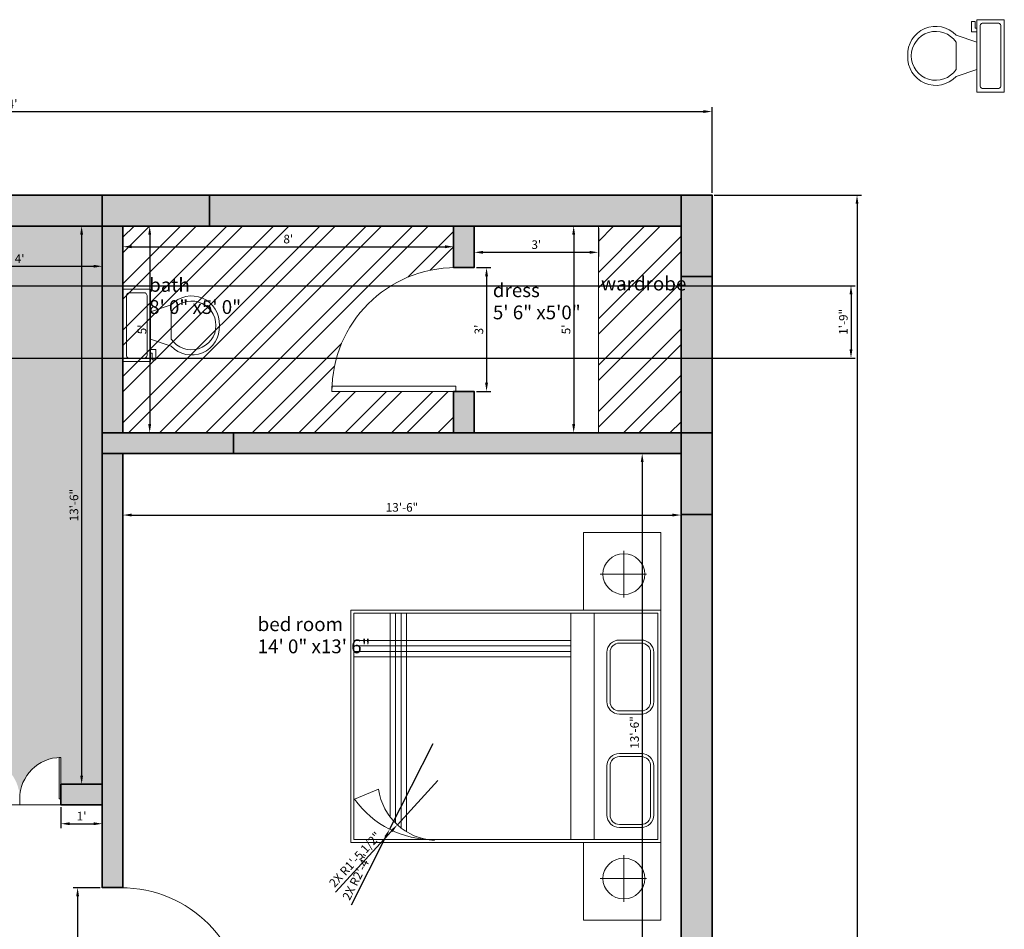
# Model space of a CAD drawing. Units: inches. Extents: x 2369 to 4208, y 1650 to 4492.
# Tile 6 of 6: x 2576 to 2862, y 2257 to 2521. Entities that reach past the tile are written whole.
import ezdxf

# ---------------------------------------------------------------- set-up
doc = ezdxf.new("R2010")
doc.units = ezdxf.units.IN
for name, color, linetype, lineweight in [('A-ANNO-DIMS', 2, 'Continuous', 13), ('A-AREA-IDEN', 7, 'Continuous', 18), ('A-COLS', 7, 'Continuous', 35), ('A-COLS-PATT', 7, 'Continuous', 13), ('A-DOOR', 4, 'Continuous', 18), ('A-FLOR-FIXT', 9, 'Continuous', 18), ('A-FLOR-PATT', 9, 'Continuous', 13), ('A-FURN', 8, 'Continuous', 18), ('A-FURN-FIXD', 8, 'Continuous', 18), ('A-WALL', 7, 'Continuous', 35), ('A-WALL-PATT', 252, 'Continuous', 13)]:
    doc.layers.add(name, color=color, linetype=linetype, lineweight=lineweight)
doc.styles.get("Standard").update_dxf_attribs({"font": 'arial.ttf'})
doc.dimstyles.new('Copy of ISO-25', dxfattribs={"dimtxt": 2.5, "dimasz": 2.5, "dimexe": 1.25, "dimexo": 0.625, "dimtad": 1, "dimdec": 1, "dimlunit": 4, "dimtxsty": 'Standard', "dimcen": 2.5, "dimadec": 0, "dimazin": 0, "dimtfac": 1, "dimtdec": 1, "dimtmove": 0, "dimatfit": 3, "dimfxl": 1, "dimarcsym": 0})

# ---------------------------------------------------------------- blocks, each defined once
blk = doc.blocks.new('*U5')
for p, q in [((0, 0), (0, -6)), ((-40, 0), (-40, -6))]:
    blk.add_line(p, q)
blk.add_lwpolyline([(0, 0), (0, 40), (-1.75, 40), (-1.75, 0)], close=True)
blk.add_arc((0, 0), 40, 90, 180)
blk = doc.blocks.new('*U4')
for p, q in [((-40, 0), (-40, 6)), ((0, 0), (0, 6))]:
    blk.add_line(p, q)
blk.add_lwpolyline([(0, 0), (0, -40), (-1.75, -40), (-1.75, 0)], close=True)
blk.add_arc((0, 0), 40, 180, 270)
blk = doc.blocks.new('*U3')
for p, q in [((0, 0), (0, -6)), ((-40, 0), (-40, -6))]:
    blk.add_line(p, q)
blk.add_lwpolyline([(0, 0), (0, 40), (-1.75, 40), (-1.75, 0)], close=True)
blk.add_arc((0, 0), 40, 90, 180)
blk = doc.blocks.new('*D7')
at = {"layer": 'A-ANNO-DIMS', "color": 0, "lineweight": -2, "transparency": 16777216}
for p, q in [((2368.9, 2470.6), (2368.9, 2495.47)), ((2776.9, 2470.6), (2776.9, 2495.47)), ((2371.4, 2494.22), (2774.4, 2494.22))]:
    blk.add_line(p, q, dxfattribs=at)
at = {"layer": 'A-ANNO-DIMS', "color": 0, "transparency": 16777216}
for points in [[(2371.4, 2494.64), (2371.4, 2493.81), (2368.9, 2494.22)], [(2774.4, 2494.64), (2774.4, 2493.81), (2776.9, 2494.22)]]:
    blk.add_solid(points, dxfattribs=at)
at = {"layer": 'Defpoints', "color": 0, "transparency": 16777216}
for p in [(2776.9, 2494.22), (2368.9, 2469.98), (2776.9, 2469.98)]:
    blk.add_point(p, dxfattribs=at)
at = {"layer": 'A-ANNO-DIMS', "color": 0, "transparency": 16777216, "insert": (2572.9, 2496.13), "char_height": 2.5, "attachment_point": 5}
blk.add_mtext("34'", dxfattribs=at)
blk = doc.blocks.new('*D8')
at = {"layer": 'A-ANNO-DIMS', "color": 0, "lineweight": -2, "transparency": 16777216}
for p, q in [((2777.53, 2469.98), (2820.25, 2469.98)), ((2819, 2467.48), (2819, 1752.48)), ((2777.53, 1749.98), (2820.25, 1749.98))]:
    blk.add_line(p, q, dxfattribs=at)
at = {"layer": 'A-ANNO-DIMS', "color": 0, "transparency": 16777216}
for points in [[(2818.58, 2467.48), (2819.41, 2467.48), (2819, 2469.98)], [(2818.58, 1752.48), (2819.41, 1752.48), (2819, 1749.98)]]:
    blk.add_solid(points, dxfattribs=at)
at = {"layer": 'Defpoints', "color": 0, "transparency": 16777216}
for p in [(2776.9, 2469.98), (2776.9, 1749.98), (2819, 1749.98)]:
    blk.add_point(p, dxfattribs=at)
at = {"layer": 'A-ANNO-DIMS', "color": 0, "transparency": 16777216, "insert": (2817.1, 2109.98), "char_height": 2.5, "attachment_point": 5, "rotation": 90}
blk.add_mtext("60'", dxfattribs=at)
blk = doc.blocks.new('*D9')
at = {"layer": 'A-ANNO-DIMS', "color": 0, "lineweight": -2, "transparency": 16777216}
for p, q in [((2551.9, 2460.35), (2551.9, 2448.06)), ((2599.9, 2460.35), (2599.9, 2448.06)), ((2554.4, 2449.31), (2597.4, 2449.31))]:
    blk.add_line(p, q, dxfattribs=at)
at = {"layer": 'A-ANNO-DIMS', "color": 0, "transparency": 16777216}
for points in [[(2554.4, 2449.73), (2554.4, 2448.9), (2551.9, 2449.31)], [(2597.4, 2449.73), (2597.4, 2448.9), (2599.9, 2449.31)]]:
    blk.add_solid(points, dxfattribs=at)
at = {"layer": 'Defpoints', "color": 0, "transparency": 16777216}
for p in [(2551.9, 2460.98), (2599.9, 2460.98), (2599.9, 2449.31)]:
    blk.add_point(p, dxfattribs=at)
at = {"layer": 'A-ANNO-DIMS', "color": 0, "transparency": 16777216, "insert": (2575.9, 2451.19), "char_height": 2.5, "attachment_point": 5}
blk.add_mtext("4'", dxfattribs=at)
blk = doc.blocks.new('*D10')
at = {"layer": 'A-ANNO-DIMS', "color": 0, "lineweight": -2, "transparency": 16777216}
for p, q in [((2599.28, 2460.98), (2592.65, 2460.98)), ((2593.9, 2458.48), (2593.9, 2301.48)), ((2599.28, 2298.98), (2592.65, 2298.98))]:
    blk.add_line(p, q, dxfattribs=at)
at = {"layer": 'A-ANNO-DIMS', "color": 0, "transparency": 16777216}
for points in [[(2593.48, 2458.48), (2594.32, 2458.48), (2593.9, 2460.98)], [(2593.48, 2301.48), (2594.32, 2301.48), (2593.9, 2298.98)]]:
    blk.add_solid(points, dxfattribs=at)
at = {"layer": 'Defpoints', "color": 0, "transparency": 16777216}
for p in [(2599.9, 2460.98), (2593.9, 2298.98), (2599.9, 2298.98)]:
    blk.add_point(p, dxfattribs=at)
at = {"layer": 'A-ANNO-DIMS', "color": 0, "transparency": 16777216, "insert": (2592, 2379.98), "char_height": 2.5, "attachment_point": 5, "rotation": 90}
blk.add_mtext('13\'-6"', dxfattribs=at)
blk = doc.blocks.new('*D15')
at = {"layer": 'A-ANNO-DIMS', "color": 0, "lineweight": -2, "transparency": 16777216}
for p, q in [((2605.9, 2460.35), (2605.9, 2453.73)), ((2701.9, 2460.35), (2701.9, 2453.73)), ((2608.4, 2454.98), (2699.4, 2454.98))]:
    blk.add_line(p, q, dxfattribs=at)
at = {"layer": 'A-ANNO-DIMS', "color": 0, "transparency": 16777216}
for points in [[(2608.4, 2455.4), (2608.4, 2454.56), (2605.9, 2454.98)], [(2699.4, 2455.4), (2699.4, 2454.56), (2701.9, 2454.98)]]:
    blk.add_solid(points, dxfattribs=at)
at = {"layer": 'Defpoints', "color": 0, "transparency": 16777216}
for p in [(2605.9, 2460.98), (2701.9, 2460.98), (2701.9, 2454.98)]:
    blk.add_point(p, dxfattribs=at)
at = {"layer": 'A-ANNO-DIMS', "color": 0, "transparency": 16777216, "insert": (2653.9, 2456.88), "char_height": 2.5, "attachment_point": 5}
blk.add_mtext("8'", dxfattribs=at)
blk = doc.blocks.new('*D16')
at = {"layer": 'A-ANNO-DIMS', "color": 0, "lineweight": -2, "transparency": 16777216}
for p, q in [((2606.53, 2460.98), (2614.91, 2460.98)), ((2613.66, 2458.48), (2613.66, 2403.48)), ((2606.53, 2400.98), (2614.91, 2400.98))]:
    blk.add_line(p, q, dxfattribs=at)
at = {"layer": 'A-ANNO-DIMS', "color": 0, "transparency": 16777216}
for points in [[(2613.24, 2458.48), (2614.08, 2458.48), (2613.66, 2460.98)], [(2613.24, 2403.48), (2614.08, 2403.48), (2613.66, 2400.98)]]:
    blk.add_solid(points, dxfattribs=at)
at = {"layer": 'Defpoints', "color": 0, "transparency": 16777216}
for p in [(2605.9, 2460.98), (2605.9, 2400.98), (2613.66, 2400.98)]:
    blk.add_point(p, dxfattribs=at)
at = {"layer": 'A-ANNO-DIMS', "color": 0, "transparency": 16777216, "insert": (2611.76, 2430.98), "char_height": 2.5, "attachment_point": 5, "rotation": 90}
blk.add_mtext("5'", dxfattribs=at)
blk = doc.blocks.new('*D17')
at = {"layer": 'A-ANNO-DIMS', "color": 0, "lineweight": -2, "transparency": 16777216}
for p, q in [((2707.9, 2460.35), (2707.9, 2452.11)), ((2743.9, 2460.35), (2743.9, 2452.11)), ((2710.4, 2453.36), (2741.4, 2453.36))]:
    blk.add_line(p, q, dxfattribs=at)
at = {"layer": 'A-ANNO-DIMS', "color": 0, "transparency": 16777216}
for points in [[(2710.4, 2453.78), (2710.4, 2452.94), (2707.9, 2453.36)], [(2741.4, 2453.78), (2741.4, 2452.94), (2743.9, 2453.36)]]:
    blk.add_solid(points, dxfattribs=at)
at = {"layer": 'Defpoints', "color": 0, "transparency": 16777216}
for p in [(2707.9, 2460.98), (2743.9, 2460.98), (2743.9, 2453.36)]:
    blk.add_point(p, dxfattribs=at)
at = {"layer": 'A-ANNO-DIMS', "color": 0, "transparency": 16777216, "insert": (2725.9, 2455.26), "char_height": 2.5, "attachment_point": 5}
blk.add_mtext("3'", dxfattribs=at)
blk = doc.blocks.new('*D18')
at = {"layer": 'A-ANNO-DIMS', "color": 0, "lineweight": -2, "transparency": 16777216}
for p, q in [((2743.28, 2460.98), (2735.49, 2460.98)), ((2736.74, 2458.48), (2736.74, 2403.48)), ((2743.28, 2400.98), (2735.49, 2400.98))]:
    blk.add_line(p, q, dxfattribs=at)
at = {"layer": 'A-ANNO-DIMS', "color": 0, "transparency": 16777216}
for points in [[(2736.32, 2458.48), (2737.16, 2458.48), (2736.74, 2460.98)], [(2736.32, 2403.48), (2737.16, 2403.48), (2736.74, 2400.98)]]:
    blk.add_solid(points, dxfattribs=at)
at = {"layer": 'Defpoints', "color": 0, "transparency": 16777216}
for p in [(2743.9, 2460.98), (2736.74, 2400.98), (2743.9, 2400.98)]:
    blk.add_point(p, dxfattribs=at)
at = {"layer": 'A-ANNO-DIMS', "color": 0, "transparency": 16777216, "insert": (2734.84, 2430.98), "char_height": 2.5, "attachment_point": 5, "rotation": 90}
blk.add_mtext("5'", dxfattribs=at)
blk = doc.blocks.new('*D21')
at = {"layer": 'A-ANNO-DIMS', "color": 0, "lineweight": -2, "transparency": 16777216}
for p, q in [((2605.9, 2394.35), (2605.9, 2375.85)), ((2767.9, 2394.35), (2767.9, 2375.85)), ((2608.4, 2377.1), (2765.4, 2377.1))]:
    blk.add_line(p, q, dxfattribs=at)
at = {"layer": 'A-ANNO-DIMS', "color": 0, "transparency": 16777216}
for points in [[(2608.4, 2377.51), (2608.4, 2376.68), (2605.9, 2377.1)], [(2765.4, 2377.51), (2765.4, 2376.68), (2767.9, 2377.1)]]:
    blk.add_solid(points, dxfattribs=at)
at = {"layer": 'Defpoints', "color": 0, "transparency": 16777216}
for p in [(2605.9, 2394.98), (2767.9, 2394.98), (2767.9, 2377.1)]:
    blk.add_point(p, dxfattribs=at)
at = {"layer": 'A-ANNO-DIMS', "color": 0, "transparency": 16777216, "insert": (2686.9, 2379), "char_height": 2.5, "attachment_point": 5}
blk.add_mtext('13\'-6"', dxfattribs=at)
blk = doc.blocks.new('*D22')
at = {"layer": 'A-ANNO-DIMS', "color": 0, "lineweight": -2, "transparency": 16777216}
for p, q in [((2767.28, 2394.98), (2755.38, 2394.98)), ((2756.63, 2392.48), (2756.63, 2235.48)), ((2767.28, 2232.98), (2755.38, 2232.98))]:
    blk.add_line(p, q, dxfattribs=at)
at = {"layer": 'A-ANNO-DIMS', "color": 0, "transparency": 16777216}
for points in [[(2756.21, 2392.48), (2757.05, 2392.48), (2756.63, 2394.98)], [(2756.21, 2235.48), (2757.05, 2235.48), (2756.63, 2232.98)]]:
    blk.add_solid(points, dxfattribs=at)
at = {"layer": 'Defpoints', "color": 0, "transparency": 16777216}
for p in [(2767.9, 2394.98), (2756.63, 2232.98), (2767.9, 2232.98)]:
    blk.add_point(p, dxfattribs=at)
at = {"layer": 'A-ANNO-DIMS', "color": 0, "transparency": 16777216, "insert": (2754.73, 2313.98), "char_height": 2.5, "attachment_point": 5, "rotation": 90}
blk.add_mtext('13\'-6"', dxfattribs=at)
blk = doc.blocks.new('A$C057D194F')
for p, q in [((0, 1.5, -0.1688), (0, 2, -0.1688)), ((0, 2, -0.1688), (0.5, 2, -0.1688)), ((0.5, 2, -0.1688), (0.5, 0, -0.1688)), ((2, 2, -0.1688), (0.5, 2, -0.1688)), ((1.98, 1.98, -0.1688), (0.52, 1.98, -0.1688)), ((0.52, 1.98, -0.1688), (0.52, 0.02, -0.1688)), ((1.98, 0.02, -0.1688), (1.98, 1.98, -0.1688)), ((2, 0, -0.1688), (2, 2, -0.1688)), ((2.5, 2, -0.1688), (2, 2, -0.1688)), ((2.5, 1.5, -0.1688), (2.5, 2, -0.1688)), ((0.2687, 1.9081, -0.1688), (0.2687, 1.761, -0.1688)), ((0.2687, 1.6081, -0.1688), (0.2687, 1.9081, -0.1688)), ((1.0907, 1.9539, -0.1688), (0.7735, 1.9539, -0.1688)), ((1.0907, 1.9339, -0.1688), (0.7735, 1.9339, -0.1688)), ((1.8224, 1.9539, -0.1688), (1.5052, 1.9539, -0.1688)), ((1.8224, 1.9339, -0.1688), (1.5052, 1.9339, -0.1688)), ((2.2313, 1.9081, -0.1688), (2.2313, 1.761, -0.1688)), ((2.2313, 1.6081, -0.1688), (2.2313, 1.9081, -0.1688)), ((0.6935, 1.8739, -0.1688), (0.6935, 1.7322, -0.1688)), ((0.7135, 1.8739, -0.1688), (0.7135, 1.7322, -0.1688)), ((1.1507, 1.7322, -0.1688), (1.1507, 1.8739, -0.1688)), ((1.1707, 1.7322, -0.1688), (1.1707, 1.8739, -0.1688)), ((1.4252, 1.8739, -0.1688), (1.4252, 1.7322, -0.1688)), ((1.4452, 1.8739, -0.1688), (1.4452, 1.7322, -0.1688)), ((1.8824, 1.7322, -0.1688), (1.8824, 1.8739, -0.1688)), ((1.9024, 1.7322, -0.1688), (1.9024, 1.8739, -0.1688)), ((0.4194, 1.761, -0.1688), (0.1194, 1.761, -0.1688)), ((0.2687, 1.761, -0.1688), (0.4194, 1.761, -0.1688)), ((0.2687, 1.761, -0.1688), (0.2687, 1.6081, -0.1688)), ((2.0806, 1.761, -0.1688), (2.3806, 1.761, -0.1688)), ((2.2313, 1.761, -0.1688), (2.0806, 1.761, -0.1688)), ((2.2313, 1.761, -0.1688), (2.2313, 1.6081, -0.1688)), ((0.7735, 1.6722, -0.1688), (1.0907, 1.6722, -0.1688)), ((0.7735, 1.6522, -0.1688), (1.0907, 1.6522, -0.1688)), ((1.5052, 1.6722, -0.1688), (1.8224, 1.6722, -0.1688)), ((1.5052, 1.6522, -0.1688), (1.8224, 1.6522, -0.1688)), ((1.98, 1.5693, -0.1688), (0.52, 1.5693, -0.1688)), ((0.5, 1.5, -0.1688), (0, 1.5, -0.1688)), ((2, 1.5, -0.1688), (2.5, 1.5, -0.1688)), ((1.98, 1.4193, -0.1688), (0.52, 1.4193, -0.1688)), ((0.6969, 0.02, -0.1688), (0.6969, 1.4193, -0.1688)), ((0.7319, 0.02, -0.1688), (0.7319, 1.4193, -0.1688)), ((0.7669, 0.02, -0.1688), (0.7669, 1.4193, -0.1688)), ((0.8019, 0.02, -0.1688), (0.8019, 1.4193, -0.1688)), ((0.52, 0.3595, -0.1688), (1.9292, 0.3595, -0.1688)), ((0.52, 0.3245, -0.1688), (1.905, 0.3245, -0.1688)), ((0.52, 0.2895, -0.1688), (1.8742, 0.2895, -0.1688)), ((0.52, 0.2545, -0.1688), (1.8344, 0.2545, -0.1688)), ((1.6548, 0.1789, -0.1688), (1.7198, 0.0251, -0.1688)), ((0.52, 0.02, -0.1688), (1.98, 0.02, -0.1688)), ((0.5, 0, -0.1688), (2, 0, -0.1688))]:
    blk.add_line(p, q)
for centre, radius, start, end in [((0.7735, 1.8739, -0.1688), 0.08, 90, 180), ((0.7735, 1.8739, -0.1688), 0.06, 90, 180), ((1.0907, 1.8739, -0.1688), 0.08, 0, 90), ((1.0907, 1.8739, -0.1688), 0.06, 0, 90), ((1.5052, 1.8739, -0.1688), 0.08, 90, 180), ((1.5052, 1.8739, -0.1688), 0.06, 90, 180), ((1.8224, 1.8739, -0.1688), 0.08, 0, 90), ((1.8224, 1.8739, -0.1688), 0.06, 0, 90), ((0.7735, 1.7322, -0.1688), 0.08, 180, 270), ((0.7735, 1.7322, -0.1688), 0.06, 180, 270), ((1.0907, 1.7322, -0.1688), 0.08, 270, 0), ((1.0907, 1.7322, -0.1688), 0.06, 270, 0), ((1.5052, 1.7322, -0.1688), 0.08, 180, 270), ((1.5052, 1.7322, -0.1688), 0.06, 180, 270), ((1.8224, 1.7322, -0.1688), 0.08, 270, 0), ((1.8224, 1.7322, -0.1688), 0.06, 270, 0), ((1.5992, 0.5623, -0.1688), 0.3874, 278.2518, 356.6808), ((1.363, 0.5286, -0.1688), 0.6171, 305.32946, 1.04595)]:
    blk.add_arc(centre, radius, start, end)
blk.add_ellipse((0.2687, 1.761, -0.1688), major_axis=(0, -0.1351), ratio=0.975448)
at = {"extrusion": (0, 0, -1)}
blk.add_ellipse((2.2313, 1.761, -0.1688), major_axis=(0, 0.1351), ratio=0.975448, dxfattribs=at)
for p in [(0.2687, 1.761, -0.1688), (2.2313, 1.761, -0.1688)]:
    blk.add_point(p)
blk = doc.blocks.new('*D40')
at = {"layer": 'A-ANNO-DIMS', "color": 0, "lineweight": -2, "transparency": 16777216}
for p, q in [((2587.9, 2292.35), (2587.9, 2286.25)), ((2599.9, 2292.35), (2599.9, 2286.25)), ((2590.4, 2287.5), (2597.4, 2287.5))]:
    blk.add_line(p, q, dxfattribs=at)
at = {"layer": 'A-ANNO-DIMS', "color": 0, "transparency": 16777216}
for points in [[(2590.4, 2287.92), (2590.4, 2287.08), (2587.9, 2287.5)], [(2597.4, 2287.92), (2597.4, 2287.08), (2599.9, 2287.5)]]:
    blk.add_solid(points, dxfattribs=at)
at = {"layer": 'Defpoints', "color": 0, "transparency": 16777216}
for p in [(2587.9, 2292.98), (2599.9, 2292.98), (2599.9, 2287.5)]:
    blk.add_point(p, dxfattribs=at)
at = {"layer": 'A-ANNO-DIMS', "color": 0, "transparency": 16777216, "insert": (2593.9, 2289.38), "char_height": 2.5, "attachment_point": 5}
blk.add_mtext("1'", dxfattribs=at)
blk = doc.blocks.new('*D41')
at = {"layer": 'A-ANNO-DIMS', "color": 0, "lineweight": -2, "transparency": 16777216}
for p, q in [((2708.53, 2448.93), (2712.7, 2448.93)), ((2711.45, 2446.43), (2711.45, 2415.48)), ((2708.53, 2412.98), (2712.7, 2412.98))]:
    blk.add_line(p, q, dxfattribs=at)
at = {"layer": 'A-ANNO-DIMS', "color": 0, "transparency": 16777216}
for points in [[(2711.03, 2446.43), (2711.87, 2446.43), (2711.45, 2448.93)], [(2711.03, 2415.48), (2711.87, 2415.48), (2711.45, 2412.98)]]:
    blk.add_solid(points, dxfattribs=at)
at = {"layer": 'Defpoints', "color": 0, "transparency": 16777216}
for p in [(2707.9, 2448.93), (2707.9, 2412.98), (2711.45, 2412.98)]:
    blk.add_point(p, dxfattribs=at)
at = {"layer": 'A-ANNO-DIMS', "color": 0, "transparency": 16777216, "insert": (2709.55, 2430.95), "char_height": 2.5, "attachment_point": 5, "rotation": 90}
blk.add_mtext("3'", dxfattribs=at)
blk = doc.blocks.new('*D43')
at = {"layer": 'A-ANNO-DIMS', "color": 0, "lineweight": -2, "transparency": 16777216}
for p, q in [((2599.28, 2268.93), (2591.48, 2268.93)), ((2592.73, 2266.43), (2592.73, 2235.48)), ((2599.28, 2232.98), (2591.48, 2232.98))]:
    blk.add_line(p, q, dxfattribs=at)
at = {"layer": 'A-ANNO-DIMS', "color": 0, "transparency": 16777216}
for points in [[(2592.31, 2266.43), (2593.15, 2266.43), (2592.73, 2268.93)], [(2592.31, 2235.48), (2593.15, 2235.48), (2592.73, 2232.98)]]:
    blk.add_solid(points, dxfattribs=at)
at = {"layer": 'Defpoints', "color": 0, "transparency": 16777216}
for p in [(2599.9, 2268.93), (2592.73, 2232.98), (2599.9, 2232.98)]:
    blk.add_point(p, dxfattribs=at)
at = {"layer": 'A-ANNO-DIMS', "color": 0, "transparency": 16777216, "insert": (2590.83, 2250.95), "char_height": 2.5, "attachment_point": 5, "rotation": 90}
blk.add_mtext("3'", dxfattribs=at)
blk = doc.blocks.new('*U47')
for p, q in [((241.3, -152.4), (241.3, -50.8)), ((-254, -215.9), (-203.2, -215.9)), ((-254, -241.3), (-254, -215.9)), ((-203.2, -215.9), (-203.2, -203.2)), ((-177.8, -203.2), (-177.8, -241.3)), ((-101.6, -203.2), (-152.4, -355.6)), ((101.6, -203.2), (152.4, -355.6)), ((-177.8, -241.3), (-254, -241.3)), ((101.6, -355.6), (-101.6, -355.6))]:
    blk.add_line(p, q)
blk.add_lwpolyline([(266.7, -203.2), (266.7, 0), (-266.7, 0), (-266.7, -203.2)], close=True)
for points in [[(-241.3, -50.8), (-241.3, -152.4)], [(215.9, -25.4), (-215.9, -25.4)], [(-215.9, -177.8), (215.9, -177.8)]]:
    blk.add_lwpolyline(points)
for centre, radius, start, end in [((-219.075, -47.625), 22.45064, 81.8699, 188.1301), ((219.075, -47.625), 22.45064, 351.8699, 98.1301), ((-219.075, -155.575), 22.45064, 171.869898, 278.1301), ((219.075, -155.575), 22.45064, 261.8699, 8.1301), ((-12.12088, -505.93752), 205.61935, 133.01722, 273.38), ((0.94996, -504.77674), 181.02486, 124.50543, 269.7), ((-0.94742, -504.77674), 181.02486, 270.3, 55.4946), ((12.12342, -505.93752), 205.61935, 266.62, 46.9828)]:
    blk.add_arc(centre, radius, start, end)
blk = doc.blocks.new('*D63')
at = {"layer": 'A-ANNO-DIMS', "color": 0, "lineweight": -2, "transparency": 16777216}
for p, q in [((2546, 2443.68), (2818.5, 2443.68)), ((2817.25, 2441.18), (2817.25, 2425.18)), ((2546, 2422.68), (2818.5, 2422.68))]:
    blk.add_line(p, q, dxfattribs=at)
at = {"layer": 'A-ANNO-DIMS', "color": 0, "transparency": 16777216}
for points in [[(2816.83, 2441.18), (2817.67, 2441.18), (2817.25, 2443.68)], [(2816.83, 2425.18), (2817.67, 2425.18), (2817.25, 2422.68)]]:
    blk.add_solid(points, dxfattribs=at)
at = {"layer": 'Defpoints', "color": 0, "transparency": 16777216}
for p in [(2545.38, 2443.68), (2545.38, 2422.68), (2817.25, 2422.68)]:
    blk.add_point(p, dxfattribs=at)
at = {"layer": 'A-ANNO-DIMS', "color": 0, "transparency": 16777216, "insert": (2815.35, 2433.18), "char_height": 2.5, "attachment_point": 5, "rotation": 90}
blk.add_mtext('1\'-9"', dxfattribs=at)
blk = doc.blocks.new('*D73')
at = {"layer": 'A-ANNO-DIMS', "color": 0, "lineweight": -2, "transparency": 16777216}
for p, q in [((2695.83, 2310.68), (2683.3, 2285.89)), ((2672.24, 2264), (2682.17, 2283.65))]:
    blk.add_line(p, q, dxfattribs=at)
at = {"layer": 'A-ANNO-DIMS', "color": 0, "transparency": 16777216}
blk.add_solid([(2681.8, 2283.84), (2682.54, 2283.47), (2683.3, 2285.89)], dxfattribs=at)
at = {"layer": 'Defpoints', "color": 0, "transparency": 16777216}
for p in [(2695.83, 2310.68), (2683.3, 2285.89)]:
    blk.add_point(p, dxfattribs=at)
at = {"layer": 'A-ANNO-DIMS', "color": 0, "transparency": 16777216, "insert": (2674.1, 2271.86), "char_height": 2.5, "attachment_point": 5, "rotation": 63.1887}
blk.add_mtext('2X R2\'-4"', dxfattribs=at)
blk = doc.blocks.new('*D74')
at = {"layer": 'A-ANNO-DIMS', "color": 0, "lineweight": -2, "transparency": 16777216}
for p, q in [((2697.35, 2300.05), (2685.56, 2287.2)), ((2667.62, 2267.65), (2683.87, 2285.35))]:
    blk.add_line(p, q, dxfattribs=at)
at = {"layer": 'A-ANNO-DIMS', "color": 0, "transparency": 16777216}
blk.add_solid([(2683.56, 2285.64), (2684.17, 2285.07), (2685.56, 2287.2)], dxfattribs=at)
at = {"layer": 'Defpoints', "color": 0, "transparency": 16777216}
for p in [(2697.35, 2300.05), (2685.56, 2287.2)]:
    blk.add_point(p, dxfattribs=at)
at = {"layer": 'A-ANNO-DIMS', "color": 0, "transparency": 16777216, "insert": (2673.49, 2276.88), "char_height": 2.5, "attachment_point": 5, "rotation": 47.4669}
blk.add_mtext('2X R1\'-5 1/2"', dxfattribs=at)

msp = doc.modelspace()

# ---------------------------------------------------------------- hatches: boundary and pattern name
at = {"layer": 'A-COLS-PATT'}
h = msp.add_hatch(color=256, dxfattribs=at)
h.dxf.hatch_style = 1
h.paths.add_polyline_path([(2377.9, 2254.21), (2368.9, 2254.21), (2368.9, 2226.98), (2377.9, 2226.98)])
h.paths.add_polyline_path([(2551.9, 2400.98), (2545.9, 2400.98), (2525.15, 2400.98), (2525.15, 2394.98), (2545.9, 2395.12), (2551.9, 2395.12)])
h.paths.add_polyline_path([(2637.99, 2400.98), (2599.9, 2400.98), (2599.9, 2394.98), (2605.9, 2394.98), (2637.99, 2394.98)])
h.paths.add_polyline_path([(2623.27, 2232.98), (2599.9, 2232.98), (2599.9, 2226.98), (2623.27, 2226.98)])
h.paths.add_polyline_path([(2551.9, 2232.98), (2528.53, 2232.98), (2528.53, 2226.98), (2551.9, 2226.98)])
h.paths.add_polyline_path([(2731.9, 2232.98), (2713.81, 2232.98), (2713.81, 2226.98), (2731.9, 2226.98)])
h.paths.add_polyline_path([(2776.9, 2250.53), (2767.9, 2250.53), (2767.9, 2232.98), (2767.9, 2226.98), (2776.9, 2226.98)])
h.paths.add_polyline_path([(2776.9, 2078.3), (2767.9, 2078.3), (2767.9, 2058.98), (2767.9, 2052.98), (2776.9, 2052.98)])
h.paths.add_polyline_path([(2731.9, 2058.98), (2725.9, 2058.98), (2713.81, 2058.98), (2713.81, 2052.98), (2731.9, 2052.98)])
h.paths.add_polyline_path([(2776.9, 1973.96), (2767.9, 1973.96), (2767.9, 1956.98), (2767.9, 1950.98), (2776.9, 1950.98)])
h.paths.add_polyline_path([(2776.9, 1775.33), (2767.9, 1775.33), (2767.9, 1758.98), (2767.9, 1749.98), (2776.9, 1749.98)])
h.paths.add_polyline_path([(2569.9, 1758.98), (2560.9, 1758.98), (2560.9, 1749.98), (2569.9, 1749.98)])
h.paths.add_polyline_path([(2377.9, 1774.03), (2368.9, 1774.03), (2368.9, 1749.98), (2372.9, 1749.98), (2377.9, 1749.98)])
h.paths.add_polyline_path([(2377.9, 1926.53), (2368.9, 1926.53), (2368.9, 1902.98), (2377.9, 1902.98)])
h.paths.add_polyline_path([(2377.9, 2079.34), (2368.9, 2079.34), (2368.9, 2052.98), (2377.9, 2052.98), (2377.9, 2057.9)])
at = {"layer": 'A-FLOR-PATT'}
h = msp.add_hatch(dxfattribs=at)
h.set_pattern_fill('ANSI32', color=256)
h.paths.add_polyline_path([(2545.9, 2460.98), (2523.46, 2460.98), (2449.9, 2460.98), (2449.9, 2448.93, -0.401453), (2485.82, 2414.55), (2485.85, 2414.55), (2485.85, 2412.98), (2449.9, 2412.98), (2449.9, 2400.98), (2545.9, 2400.98)])
h.paths.add_polyline_path([(2701.9, 2448.92), (2701.9, 2460.98), (2605.9, 2460.98), (2605.9, 2400.98), (2637.99, 2400.98), (2701.9, 2400.98), (2701.9, 2412.98), (2666.56, 2412.98), (2666.56, 2414.55), (2666.59, 2414.55, -0.396556)])
h.paths.add_polyline_path([(2425.9, 2148.98), (2377.9, 2148.98), (2377.9, 2090.68), (2379.33, 2090.68), (2379.33, 2090.65, -0.391899), (2410.67, 2058.98), (2425.9, 2058.98), (2425.9, 2094.98), (2425.9, 2100.98)])
h.paths.add_polyline_path([(2401.9, 2460.98), (2377.9, 2460.98), (2377.9, 2400.98), (2401.9, 2400.98)])
h.paths.add_polyline_path([(2767.9, 2460.98), (2743.9, 2460.98), (2743.9, 2400.98), (2767.9, 2400.98)])
h.paths.add_polyline_path([(2767.9, 2226.98), (2731.9, 2226.98), (2731.9, 2058.98), (2767.9, 2058.98)])
h.paths.add_polyline_path([(2612.47, 2434.38), (2640.5, 2434.38), (2640.5, 2440.51), (2612.47, 2440.51)], flags=24)
h.paths.add_polyline_path([(2612.48, 2440.81), (2625.39, 2440.81), (2625.39, 2446.91), (2612.48, 2446.91)], flags=24)
h.paths.add_polyline_path([(2712.27, 2432.83), (2738.74, 2432.83), (2738.74, 2438.96), (2712.27, 2438.96)], flags=9)
h.paths.add_polyline_path([(2712.27, 2439.27), (2727.97, 2439.27), (2727.97, 2445.37), (2712.27, 2445.37)], flags=9)
h.paths.add_polyline_path([(2492.48, 2432.36), (2520.5, 2432.36), (2520.5, 2438.49), (2492.48, 2438.49)], flags=24)
h.paths.add_polyline_path([(2492.48, 2438.8), (2505.39, 2438.8), (2505.39, 2444.9), (2492.48, 2444.9)], flags=24)
h.paths.add_polyline_path([(2386, 2119.22), (2414.03, 2119.22), (2414.03, 2125.35), (2386, 2125.35)], flags=24)
h.paths.add_polyline_path([(2386.01, 2125.66), (2398.92, 2125.66), (2398.92, 2131.75), (2386.01, 2131.75)], flags=24)
h.paths.add_polyline_path([(2377.88, 2440.75), (2403.21, 2440.75), (2403.21, 2446.85), (2377.88, 2446.85)], flags=9)
h.paths.add_polyline_path([(2743.66, 2441.21), (2768.99, 2441.21), (2768.99, 2447.31), (2743.66, 2447.31)], flags=9)
h.paths.add_polyline_path([(2739.13, 2166.12), (2752.65, 2166.12), (2752.65, 2172.22), (2739.13, 2172.22)], flags=24)
h.paths.add_polyline_path([(2739.12, 2172.54), (2751.98, 2172.54), (2751.98, 2178.67), (2739.12, 2178.67)], flags=24)
h.paths.add_polyline_path([(2738.85, 2177.59), (2749.82, 2177.59), (2749.82, 2185.35), (2738.85, 2185.35)], flags=24)
h.paths.add_polyline_path([(2739.15, 2185.42), (2747.35, 2185.42), (2747.35, 2191.39), (2739.15, 2191.39)], flags=24)
h.paths.add_polyline_path([(2739.12, 2190.78), (2753.59, 2190.78), (2753.59, 2196.89), (2739.12, 2196.89)], flags=24)
h = msp.add_hatch(dxfattribs=at)
h.set_pattern_fill('ANGLE', color=256)
h.set_pattern_definition([(0, (0, 0), (0, 6.985), [5.08, -1.905]), (90, (0, 0), (-6.985, 4e-16), [5.08, -1.905])])
h.paths.add_polyline_path([(2599.9, 2460.98), (2551.9, 2460.98), (2551.9, 2298.98), (2563.9, 2298.98), (2563.9, 2306.63), (2564.42, 2306.63), (2564.42, 2306.61, -0.405418), (2575.94, 2294.77, -0.401619), (2587.38, 2306.72), (2587.38, 2306.73), (2587.9, 2306.73), (2587.9, 2298.98), (2599.9, 2298.98)])
h.paths.add_polyline_path([(2425.9, 2226.98), (2377.9, 2226.98), (2377.9, 2154.98), (2389.9, 2154.98), (2425.9, 2154.98)])
h.paths.add_polyline_path([(2641.9, 2052.98), (2569.9, 2052.98), (2569.9, 1998.98), (2581.9, 1998.98), (2581.9, 1992.98), (2606.44, 1992.98), (2629.9, 1992.98), (2629.9, 1998.98), (2641.9, 1998.98), (2641.9, 2008.36), (2647.9, 2008.36), (2647.9, 1956.98), (2767.9, 1956.98), (2767.9, 2052.98), (2647.9, 2052.98), (2647.9, 2044.36), (2641.9, 2044.36)])
h.paths.add_polyline_path([(2628.69, 2019.73), (2629.71, 2019.73), (2629.71, 1996.47), (2628.69, 1996.47)], flags=16)
h.paths.add_polyline_path([(2563.51, 2406.86), (2576.05, 2406.86), (2576.05, 2412.82), (2563.51, 2412.82)], flags=24)
h.paths.add_polyline_path([(2391.33, 2190.25), (2403.87, 2190.25), (2403.87, 2196.21), (2391.33, 2196.21)], flags=24)
h.paths.add_polyline_path([(2704.89, 2039.23), (2710.69, 2039.23), (2710.69, 2044.38), (2704.89, 2044.38)], flags=24)
h.paths.add_polyline_path([(2759.77, 2003.06), (2759.77, 2006.92), (2754.62, 2006.92), (2754.62, 2003.06)], flags=24)
h.paths.add_polyline_path([(2707.15, 2003.75), (2738.28, 2003.75), (2738.28, 2009.88), (2707.15, 2009.88)], flags=24)
h.paths.add_polyline_path([(2707.15, 2010.19), (2726.89, 2010.19), (2726.89, 2016.29), (2707.15, 2016.29)], flags=24)
h.paths.add_polyline_path([(2577.31, 2031), (2605.34, 2031), (2605.34, 2037.12), (2577.31, 2037.12)], flags=24)
h.paths.add_polyline_path([(2577.02, 2036.02), (2603.33, 2036.02), (2603.33, 2043.89), (2577.02, 2043.89)], flags=24)
at = {"layer": 'A-WALL-PATT'}
h = msp.add_hatch(color=256, dxfattribs=at)
h.dxf.hatch_style = 1
h.paths.add_polyline_path([(2377.9, 2052.98), (2368.9, 2052.98), (2368.9, 1926.53), (2377.9, 1926.53)])
h.paths.add_polyline_path([(2377.9, 2226.98), (2368.9, 2226.98), (2368.9, 2079.34), (2377.9, 2079.34)])
h.paths.add_polyline_path([(2377.9, 2394.98), (2377.9, 2460.98), (2767.9, 2460.98), (2767.9, 2250.53), (2776.9, 2250.53), (2776.9, 2469.98), (2368.9, 2469.98), (2368.9, 2254.21), (2377.9, 2254.21)])
h.paths.add_polyline_path([(2776.9, 2226.98), (2767.9, 2226.98), (2767.9, 2078.3), (2776.9, 2078.3)])
h.paths.add_polyline_path([(2776.9, 2052.98), (2767.9, 2052.98), (2767.9, 1973.96), (2776.9, 1973.96)])
h.paths.add_polyline_path([(2776.9, 1950.98), (2767.9, 1950.98), (2767.9, 1775.33), (2776.9, 1775.33)])
h.paths.add_polyline_path([(2560.9, 1758.98), (2377.9, 1758.98), (2377.9, 1749.98), (2386.24, 1749.98), (2386.07, 1750.89), (2387.22, 1749.98), (2560.9, 1749.98)])
h.paths.add_polyline_path([(2377.9, 1902.98), (2368.9, 1902.98), (2368.9, 1774.03), (2377.9, 1774.03)])
h.paths.add_polyline_path([(2569.9, 1908.98), (2569.9, 1944.98), (2563.9, 1944.98), (2563.9, 1908.98), (2377.9, 1908.98), (2377.9, 1902.98), (2569.9, 1902.98)])
h.paths.add_polyline_path([(2523.29, 2058.98), (2411, 2058.98), (2411, 2052.98), (2523.29, 2052.98)])
h.paths.add_polyline_path([(2569.9, 2052.98), (2641.9, 2052.98), (2713.81, 2052.98), (2713.81, 2058.98), (2559.29, 2058.98), (2559.29, 2052.98), (2563.9, 2052.98), (2563.9, 1980.98), (2569.9, 1980.98), (2569.9, 1992.98)])
h.paths.add_polyline_path([(2528.53, 2232.98), (2510.56, 2232.98), (2377.9, 2232.98), (2377.9, 2226.98), (2528.53, 2226.98)])
h.paths.add_polyline_path([(2713.81, 2232.98), (2623.27, 2232.98), (2623.27, 2226.98), (2713.81, 2226.98)])
h.paths.add_polyline_path([(2647.9, 2008.36), (2642.51, 2008.36), (2641.9, 2008.36), (2641.9, 1956.98), (2641.9, 1950.98), (2767.9, 1950.98), (2767.9, 1956.98), (2647.9, 1956.98)])
h.paths.add_polyline_path([(2551.9, 2395.12), (2545.9, 2395.12), (2545.9, 2268.98), (2551.9, 2268.98)], flags=17)
h.paths.add_polyline_path([(2551.9, 2460.98), (2545.9, 2460.98), (2545.9, 2400.98), (2551.9, 2400.98)], flags=17)
h.paths.add_polyline_path([(2605.9, 2460.98), (2599.9, 2460.98), (2599.9, 2400.98), (2605.9, 2400.98)], flags=17)
h.paths.add_polyline_path([(2767.9, 2400.98), (2637.99, 2400.98), (2637.99, 2394.98), (2767.9, 2394.98)], flags=17)
h.paths.add_polyline_path([(2605.9, 2394.98), (2599.9, 2394.98), (2599.9, 2394.42), (2599.9, 2268.98), (2605.9, 2268.98)], flags=17)
h.paths.add_polyline_path([(2525.15, 2400.98), (2377.9, 2400.98), (2377.9, 2394.98), (2525.15, 2394.98)], flags=17)
h.paths.add_polyline_path([(2449.9, 2412.98), (2444.51, 2412.98), (2443.9, 2412.98), (2443.9, 2400.98), (2449.9, 2400.98)], flags=17)
h.paths.add_polyline_path([(2449.9, 2460.98), (2443.9, 2460.98), (2443.9, 2448.98), (2449.9, 2448.98)], flags=17)
h.paths.add_polyline_path([(2731.9, 2106.98), (2725.9, 2106.98), (2725.9, 2058.98), (2731.9, 2058.98)])
h = msp.add_hatch(color=256, dxfattribs=at)
h.dxf.hatch_style = 1
h.paths.add_polyline_path([(2707.9, 2412.98), (2702.51, 2412.98), (2701.9, 2412.98), (2701.9, 2400.98), (2707.9, 2400.98)])
h.paths.add_polyline_path([(2707.9, 2460.98), (2701.9, 2460.98), (2701.9, 2448.98), (2707.9, 2448.98)])
h = msp.add_hatch(color=256, dxfattribs=at)
h.dxf.hatch_style = 1
h.paths.add_polyline_path([(2563.9, 2294.76), (2563.9, 2298.98), (2551.9, 2298.98), (2551.9, 2292.98), (2563.9, 2292.98)])
h.paths.add_polyline_path([(2599.9, 2298.98), (2587.9, 2298.98), (2587.9, 2294.77), (2587.9, 2292.98), (2599.9, 2292.98)])

# ---------------------------------------------------------------- linework, layer by layer
at = {"layer": 'A-COLS'}
for p, q in [((2599.9, 2460.98), (2599.9, 2469.98)), ((2599.9, 2469.98), (2630.99, 2469.98)), ((2630.99, 2469.98), (2630.99, 2460.98)), ((2767.9, 2460.98), (2767.9, 2469.98)), ((2767.9, 2460.98), (2767.9, 2446.33)), ((2767.9, 2446.33), (2776.9, 2446.33)), ((2637.99, 2400.98), (2599.9, 2400.98)), ((2599.9, 2400.98), (2599.9, 2394.42)), ((2637.99, 2394.98), (2637.99, 2400.98)), ((2767.9, 2400.98), (2776.9, 2400.98)), ((2776.9, 2400.98), (2776.9, 2377.3)), ((2605.9, 2394.98), (2599.9, 2394.98)), ((2605.9, 2394.98), (2637.99, 2394.98)), ((2776.9, 2377.3), (2767.9, 2377.3))]:
    msp.add_line(p, q, dxfattribs=at)
at = {"layer": 'A-DOOR'}
msp.add_line((2563.9, 2292.98), (2587.9, 2292.98), dxfattribs=at)
at = {"layer": 'A-FURN-FIXD'}
for p, q in [((2767.9, 2460.98), (2743.9, 2460.98)), ((2743.9, 2460.98), (2743.9, 2400.98))]:
    msp.add_line(p, q, dxfattribs=at)
at = {"layer": 'A-WALL'}
for p, q in [((2551.9, 2460.98), (2599.9, 2460.98)), ((2599.9, 2460.98), (2599.9, 2268.98)), ((2605.9, 2460.98), (2701.9, 2460.98)), ((2605.9, 2400.98), (2605.9, 2460.98)), ((2701.9, 2460.98), (2701.9, 2448.98)), ((2707.9, 2460.98), (2707.9, 2448.98)), ((2707.9, 2448.98), (2707.9, 2460.98)), ((2707.9, 2448.98), (2701.9, 2448.98)), ((2707.9, 2412.98), (2701.9, 2412.98)), ((2701.9, 2412.98), (2701.9, 2400.98)), ((2707.9, 2400.98), (2707.9, 2412.98)), ((2767.9, 2400.98), (2605.9, 2400.98)), ((2701.9, 2400.98), (2707.9, 2400.98)), ((2605.9, 2268.98), (2605.9, 2394.98)), ((2605.9, 2394.98), (2767.9, 2394.98)), ((2587.9, 2292.98), (2587.9, 2298.98)), ((2587.9, 2298.98), (2599.9, 2298.98)), ((2599.9, 2292.98), (2587.9, 2292.98)), ((2587.9, 2292.98), (2599.9, 2292.98)), ((2599.9, 2268.98), (2605.9, 2268.98)), ((2599.9, 2268.98), (2599.9, 2268.93))]:
    msp.add_line(p, q, dxfattribs=at)
for points in [[(2368.9, 1749.98), (2368.9, 2469.98), (2776.9, 2469.98), (2776.9, 1749.98), (2689.9, 1749.98)], [(2767.9, 2052.98), (2767.9, 1758.98), (2377.9, 1758.98), (2377.9, 2460.98), (2767.9, 2460.98), (2767.9, 2232.98)]]:
    msp.add_lwpolyline(points, dxfattribs=at)

# ---------------------------------------------------------------- block references
at = {"layer": 'A-DOOR', "xscale": 0.8987594980764617, "yscale": 0.8987594980764617, "zscale": 0.8987594980764617, "rotation": 270}
for name, p in [('*U4', (2702.51, 2412.98)), ('*U5', (2605.29, 2232.98))]:
    msp.add_blockref(name, p, dxfattribs=at)
at = {"layer": 'A-DOOR', "xscale": 0.2989603819170715, "yscale": 0.2989603819170715, "zscale": 0.2989603819170715}
msp.add_blockref('*U3', (2587.9, 2294.77), dxfattribs=at)
at = {"layer": 'A-FLOR-FIXT', "xscale": 0.0393700787401575, "yscale": 0.0393700787401575, "zscale": 0.0393700787401575}
for p, rotation in [((2861.75, 2510.39), 270), ((2605.9, 2432.13), 90)]:
    msp.add_blockref('*U47', p, dxfattribs=dict(at, rotation=rotation))
at = {"layer": 'A-FURN', "xscale": 45.01703552962593, "yscale": 45.01703552962593, "zscale": 45.01703552962593, "rotation": 270}
msp.add_blockref('A$C057D194F', (2672.03, 2372.04, 7.6), dxfattribs=at)

# ---------------------------------------------------------------- texts
at = {"layer": 'A-AREA-IDEN'}
for s, p in [('bath', (2613.49, 2441.9)), ('dress', (2713.29, 2440.35)), ('wardrobe', (2744.68, 2442.29)), ('8\' 0" x5\' 0"', (2613.49, 2435.47)), ('5\' 6" x5\'0"', (2713.29, 2433.92)), ('bed room', (2645, 2343.41)), ('14\' 0" x13\' 6"', (2645, 2336.98))]:
    msp.add_text(s, height=4, dxfattribs=at).set_placement(p)

# ---------------------------------------------------------------- dimensions: what is measured, and where the dimension line sits
at = {"layer": 'A-ANNO-DIMS'}
for base, p1, p2, picture, middle in [((2776.9, 2494.22), (2368.9, 2469.98), (2776.9, 2469.98), '*D7', (2572.9, 2496.13)), ((2599.9, 2449.31), (2551.9, 2460.98), (2599.9, 2460.98), '*D9', (2575.9, 2451.19)), ((2701.9, 2454.98), (2605.9, 2460.98), (2701.9, 2460.98), '*D15', (2653.9, 2456.88)), ((2743.9, 2453.36), (2707.9, 2460.98), (2743.9, 2460.98), '*D17', (2725.9, 2455.26)), ((2767.9, 2377.1), (2605.9, 2394.98), (2767.9, 2394.98), '*D21', (2686.9, 2379)), ((2599.9, 2287.5), (2587.9, 2292.98), (2599.9, 2292.98), '*D40', (2593.9, 2289.38))]:
    dim = msp.add_linear_dim(base=base, p1=p1, p2=p2, dimstyle='Copy of ISO-25', override={"dimclrd": 0, "dimclre": 0, "dimclrt": 0}, dxfattribs=at)
    dim.commit()
    dim.dimension.update_dxf_attribs({"geometry": picture, "text_midpoint": middle})
for base, p1, p2, override, picture, middle in [((2819, 1749.98), (2776.9, 2469.98), (2776.9, 1749.98), {"dimclrd": 0, "dimclre": 0, "dimclrt": 0}, '*D8', (2817.1, 2109.98)), ((2593.9, 2298.98), (2599.9, 2460.98), (2599.9, 2298.98), {"dimclrd": 0, "dimclre": 0, "dimclrt": 0}, '*D10', (2592, 2379.98)), ((2613.66, 2400.98), (2605.9, 2460.98), (2605.9, 2400.98), {"dimclrd": 0, "dimclre": 0, "dimclrt": 0}, '*D16', (2611.76, 2430.98)), ((2736.74, 2400.98), (2743.9, 2460.98), (2743.9, 2400.98), {"dimclrd": 0, "dimclre": 0, "dimclrt": 0}, '*D18', (2734.84, 2430.98)), ((2711.4484, 2412.9785), (2707.9004, 2448.9289), (2707.9004, 2412.9785), {"dimclrd": 0, "dimclre": 0, "dimclrt": 0}, '*D41', (2709.5461, 2430.9537)), ((2817.25, 2422.68), (2545.38, 2443.68), (2545.38, 2422.68), {"dimdec": 1, "dimlfac": 1, "dimrnd": 0, "dimzin": 1, "dimdsep": 46, "dimlunit": 4, "dimfrac": 2}, '*D63', (2815.35, 2433.18)), ((2756.63, 2232.98), (2767.9, 2394.98), (2767.9, 2232.98), {"dimclrd": 0, "dimclre": 0, "dimclrt": 0}, '*D22', (2754.73, 2313.98)), ((2592.7288, 2232.9785), (2599.9004, 2268.9289), (2599.9004, 2232.9785), {"dimclrd": 0, "dimclre": 0, "dimclrt": 0}, '*D43', (2590.8265, 2250.9537))]:
    dim = msp.add_linear_dim(base=base, p1=p1, p2=p2, angle=90, dimstyle='Copy of ISO-25', override=override, dxfattribs=at)
    dim.commit()
    dim.dimension.update_dxf_attribs({"geometry": picture, "text_midpoint": middle})
dim = msp.add_radius_dim(center=(2695.83, 2310.68), mpoint=(2683.3, 2285.89), text='2X <>', dimstyle='Copy of ISO-25', override={"dimdec": 1, "dimlfac": 1, "dimrnd": 0, "dimzin": 1, "dimdsep": 46, "dimlunit": 4, "dimfrac": 2}, dxfattribs=at)
dim.commit()
dim.dimension.update_dxf_attribs({"geometry": '*D73', "text_midpoint": (2675.78, 2271.01), "dimtype": 164})
dim = msp.add_radius_dim(center=(2697.35, 2300.05), mpoint=(2685.56, 2287.2), text='2X <>', dimstyle='Copy of ISO-25', override={"dimdec": 1, "dimlfac": 1, "dimrnd": 0, "dimzin": 1, "dimdsep": 46, "dimlunit": 4, "dimfrac": 2}, dxfattribs=at)
dim.commit()
dim.dimension.update_dxf_attribs({"geometry": '*D74', "text_midpoint": (2673.49, 2276.88)})

doc.saveas('drawing.dxf')
